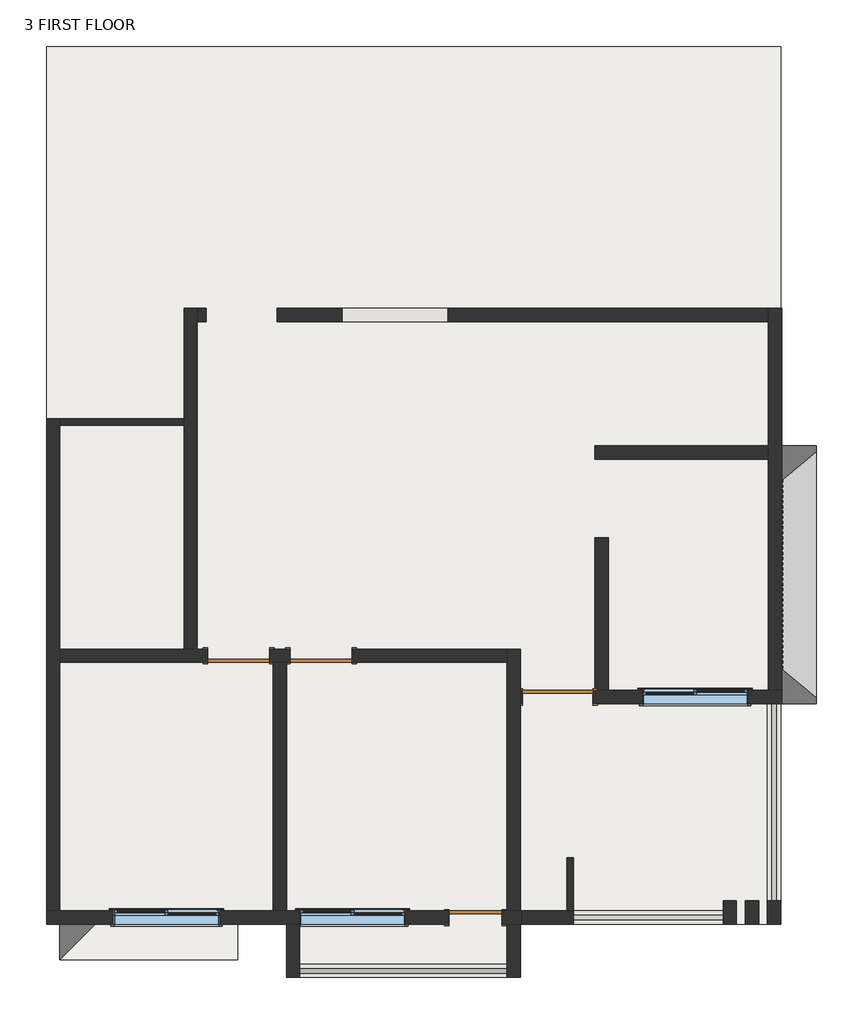
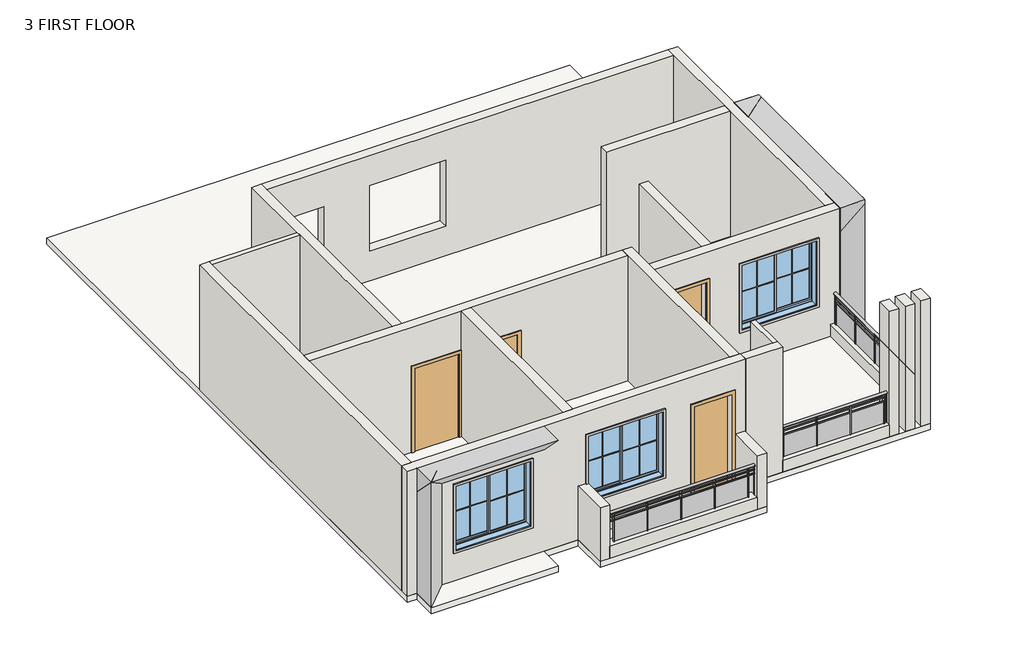
# One storey: 22 walls, 14 proxies, 4 doors, 3 railings, 3 windows, 1 slab.
"""IFC4 building model written with IfcOpenShell, lengths in millimetres."""

from ifc_helpers import new_model, si_unit, point, frame, origin, place, context, project, spatial, polyline, ellipse_curve, trimmed, outline, extrude, faceted_brep, transform, mapped, element, save
from ifc_brep_helpers import plane_surface, extruded_surface, advanced_brep
from components import generic_models_2_generic_models_2_bb9d770e, generic_models_4_generic_models_4_3dac0b09, muntin_pattern_2x2_muntin_pattern_2x2_52b72501, muntin_pattern_2x2_muntin_pattern_2x2_a6e57790, trim_window_exterior_flat_with_sill_c98b2dec, trim_window_exterior_flat_with_sill_2360300c, trim_window_interior_flat_picture_frame_b05ee221, trim_window_interior_flat_picture_frame_67c405d8, single_flush_9d399b00, single_flush_0848dd25, single_flush_md_e3fbe821, single_flush_md_2_408f135a, window_sliding_double_89c6b595, window_sliding_double_c634d93e

model = new_model("IFC4")

# Units and contexts
model_context = context("Model", 3, world=origin())
ifc_project = project(units=[si_unit("LENGTHUNIT", "METRE", prefix="MILLI")], contexts=[model_context])

# Site, building, storey
site = spatial("IfcSite", under=ifc_project)
building = spatial("IfcBuilding", under=site)
storey = spatial("IfcBuildingStorey", under=building, Name="3 FIRST FLOOR", Elevation=3505.2)

# Proxies
placement = place(None, origin())
generic_models_2_generic_models_2_shape = generic_models_2_generic_models_2_bb9d770e(model_context)
element("IfcBuildingElementProxy", 1, Name="Generic Models 2 : Generic Models 2", ObjectType="Generic Models 2 : Generic Models 2", at=placement, inside=storey, context=model_context, shape_type="MappedRepresentation", body=[
    mapped(generic_models_2_generic_models_2_shape, transform((0.0, 0.0, 0.0), x_axis=(1.0, 0.0, 0.0), y_axis=(0.0, 1.0, 0.0), z_axis=(0.0, 0.0, 1.0))),
])
generic_models_4_generic_models_4_shape = generic_models_4_generic_models_4_3dac0b09(model_context)
element("IfcBuildingElementProxy", 2, Name="Generic Models 4 : Generic Models 4", ObjectType="Generic Models 4 : Generic Models 4", at=placement, inside=storey, context=model_context, shape_type="MappedRepresentation", body=[
    mapped(generic_models_4_generic_models_4_shape, transform((0.0, 0.0, 0.0), x_axis=(1.0, 0.0, 0.0), y_axis=(0.0, 1.0, 0.0), z_axis=(0.0, 0.0, 1.0))),
])
muntin_pattern_2x2_muntin_pattern_2x2_shape = muntin_pattern_2x2_muntin_pattern_2x2_52b72501(model_context)
element("IfcBuildingElementProxy", 3, Name="Muntin Pattern_2x2 : Muntin Pattern_2x2", ObjectType="Muntin Pattern_2x2 : Muntin Pattern_2x2", at=placement, inside=storey, context=model_context, shape_type="MappedRepresentation", body=[
    mapped(muntin_pattern_2x2_muntin_pattern_2x2_shape, transform((-2582.8521564, -7786.433484, 4349.75), x_axis=(1.0, 0.0, 0.0), y_axis=(0.0, 1.0, 0.0), z_axis=(0.0, 0.0, 1.0))),
])
element("IfcBuildingElementProxy", 4, Name="Muntin Pattern_2x2 : Muntin Pattern_2x2", ObjectType="Muntin Pattern_2x2 : Muntin Pattern_2x2", at=placement, inside=storey, context=model_context, shape_type="MappedRepresentation", body=[
    mapped(muntin_pattern_2x2_muntin_pattern_2x2_shape, transform((-3455.9771564, -7741.983484, 4349.75), x_axis=(1.0, 0.0, 0.0), y_axis=(0.0, 1.0, 0.0), z_axis=(0.0, 0.0, 1.0))),
])
element("IfcBuildingElementProxy", 5, Name="Muntin Pattern_2x2 : Muntin Pattern_2x2", ObjectType="Muntin Pattern_2x2 : Muntin Pattern_2x2", at=placement, inside=storey, context=model_context, shape_type="MappedRepresentation", body=[
    mapped(muntin_pattern_2x2_muntin_pattern_2x2_shape, transform((618.6182451, -7786.433484, 4502.15), x_axis=(1.0, 0.0, 0.0), y_axis=(0.0, 1.0, 0.0), z_axis=(0.0, 0.0, 1.0))),
])
element("IfcBuildingElementProxy", 6, Name="Muntin Pattern_2x2 : Muntin Pattern_2x2", ObjectType="Muntin Pattern_2x2 : Muntin Pattern_2x2", at=placement, inside=storey, context=model_context, shape_type="MappedRepresentation", body=[
    mapped(muntin_pattern_2x2_muntin_pattern_2x2_shape, transform((-254.5067549, -7741.983484, 4502.15), x_axis=(1.0, 0.0, 0.0), y_axis=(0.0, 1.0, 0.0), z_axis=(0.0, 0.0, 1.0))),
])
muntin_pattern_2x2_muntin_pattern_2x2_2_shape = muntin_pattern_2x2_muntin_pattern_2x2_a6e57790(model_context)
element("IfcBuildingElementProxy", 7, Name="Muntin Pattern_2x2 : Muntin Pattern_2x2", ObjectType="Muntin Pattern_2x2 : Muntin Pattern_2x2", at=placement, inside=storey, context=model_context, shape_type="MappedRepresentation", body=[
    mapped(muntin_pattern_2x2_muntin_pattern_2x2_2_shape, transform((5644.6432451, -3992.2046941, 4502.15), x_axis=(-1.0, 0.0, 0.0), y_axis=(0.0, -1.0, 0.0), z_axis=(0.0, 0.0, 1.0))),
])
element("IfcBuildingElementProxy", 8, Name="Muntin Pattern_2x2 : Muntin Pattern_2x2", ObjectType="Muntin Pattern_2x2 : Muntin Pattern_2x2", at=placement, inside=storey, context=model_context, shape_type="MappedRepresentation", body=[
    mapped(muntin_pattern_2x2_muntin_pattern_2x2_2_shape, transform((6517.7682451, -3947.7546941, 4502.15), x_axis=(-1.0, 0.0, 0.0), y_axis=(0.0, -1.0, 0.0), z_axis=(0.0, 0.0, 1.0))),
])
trim_window_exterior_flat_with_sill_shape = trim_window_exterior_flat_with_sill_c98b2dec(model_context)
element("IfcBuildingElementProxy", 9, Name="Trim-Window-Exterior-Flat : with Sill", ObjectType="Trim-Window-Exterior-Flat : with Sill", at=placement, inside=storey, context=model_context, shape_type="MappedRepresentation", body=[
    mapped(trim_window_exterior_flat_with_sill_shape, transform((-3019.4146564, -7732.458484, 5943.6), x_axis=(-1.0, 0.0, 0.0), y_axis=(0.0, 0.0, 1.0), z_axis=(0.0, 1.0, 0.0))),
])
element("IfcBuildingElementProxy", 10, Name="Trim-Window-Exterior-Flat : with Sill", ObjectType="Trim-Window-Exterior-Flat : with Sill", at=placement, inside=storey, context=model_context, shape_type="MappedRepresentation", body=[
    mapped(trim_window_exterior_flat_with_sill_shape, transform((182.0557451, -7732.458484, 6096.0), x_axis=(-1.0, 0.0, 0.0), y_axis=(0.0, 0.0, 1.0), z_axis=(0.0, 1.0, 0.0))),
])
trim_window_exterior_flat_with_sill_2_shape = trim_window_exterior_flat_with_sill_2360300c(model_context)
element("IfcBuildingElementProxy", 11, Name="Trim-Window-Exterior-Flat : with Sill", ObjectType="Trim-Window-Exterior-Flat : with Sill", at=placement, inside=storey, context=model_context, shape_type="MappedRepresentation", body=[
    mapped(trim_window_exterior_flat_with_sill_2_shape, transform((6081.2057451, -3938.2296941, 6096.0), x_axis=(1.0, 0.0, 0.0), y_axis=(0.0, 0.0, -1.0), z_axis=(0.0, 1.0, 0.0))),
])
trim_window_interior_flat_picture_frame_shape = trim_window_interior_flat_picture_frame_b05ee221(model_context)
element("IfcBuildingElementProxy", 12, Name="Trim-Window-Interior-Flat : Picture Frame", ObjectType="Trim-Window-Interior-Flat : Picture Frame", at=placement, inside=storey, context=model_context, shape_type="MappedRepresentation", body=[
    mapped(trim_window_interior_flat_picture_frame_shape, transform((-3019.4146564, -7961.058484, 5943.6), x_axis=(1.0, 0.0, 0.0), y_axis=(0.0, 0.0, 1.0), z_axis=(0.0, -1.0, 0.0))),
])
element("IfcBuildingElementProxy", 13, Name="Trim-Window-Interior-Flat : Picture Frame", ObjectType="Trim-Window-Interior-Flat : Picture Frame", at=placement, inside=storey, context=model_context, shape_type="MappedRepresentation", body=[
    mapped(trim_window_interior_flat_picture_frame_shape, transform((182.0557451, -7961.058484, 6096.0), x_axis=(1.0, 0.0, 0.0), y_axis=(0.0, 0.0, 1.0), z_axis=(0.0, -1.0, 0.0))),
])
trim_window_interior_flat_picture_frame_2_shape = trim_window_interior_flat_picture_frame_67c405d8(model_context)
element("IfcBuildingElementProxy", 14, Name="Trim-Window-Interior-Flat : Picture Frame", ObjectType="Trim-Window-Interior-Flat : Picture Frame", at=placement, inside=storey, context=model_context, shape_type="MappedRepresentation", body=[
    mapped(trim_window_interior_flat_picture_frame_2_shape, transform((6081.2057451, -4166.8296941, 6096.0), x_axis=(-1.0, 0.0, 0.0), y_axis=(0.0, 0.0, -1.0), z_axis=(0.0, -1.0, 0.0))),
])

# Doors
single_flush_shape = single_flush_9d399b00(model_context)
element("IfcDoor", 15, ObjectType="Single-Flush", at=placement, inside=storey, context=model_context, shape_type="MappedRepresentation", body=[
    mapped(single_flush_shape, transform((-357.6942549, -3341.3296941, 3505.2), x_axis=(-1.0, 0.0, 0.0), y_axis=(0.0, -1.0, 0.0), z_axis=(0.0, 0.0, 1.0))),
])
single_flush_2_shape = single_flush_0848dd25(model_context)
element("IfcDoor", 16, ObjectType="Single-Flush", at=placement, inside=storey, context=model_context, shape_type="MappedRepresentation", body=[
    mapped(single_flush_2_shape, transform((-1780.0942549, -3341.3296941, 3505.2), x_axis=(1.0, 0.0, 0.0), y_axis=(0.0, 1.0, 0.0), z_axis=(0.0, 0.0, 1.0))),
])
single_flush_md_shape = single_flush_md_e3fbe821(model_context)
element("IfcDoor", 17, ObjectType="Single-Flush : MD", at=placement, inside=storey, context=model_context, shape_type="MappedRepresentation", body=[
    mapped(single_flush_md_shape, transform((3712.6557451, -4052.5296941, 3505.2), x_axis=(1.0, 0.0, 0.0), y_axis=(0.0, 1.0, 0.0), z_axis=(0.0, 0.0, 1.0))),
])
single_flush_md_2_shape = single_flush_md_2_408f135a(model_context)
element("IfcDoor", 18, ObjectType="Single-Flush : MD 2", at=placement, inside=storey, context=model_context, shape_type="MappedRepresentation", body=[
    mapped(single_flush_md_2_shape, transform((2296.6057451, -7846.758484, 3505.2), x_axis=(1.0, 0.0, 0.0), y_axis=(0.0, 1.0, 0.0), z_axis=(0.0, 0.0, 1.0))),
])

# Railings
element("IfcRailing", 19, ObjectType="Glass Panel - Bottom Fill", at=placement, inside=storey, context=model_context, shape_type="SolidModel", body=[
    advanced_brep(
    [(-725.9942549, -8723.058484, 4572.0), (-725.9942549, -8799.258484, 4572.0), (2842.7057451, -8723.058484, 4572.0), (2842.7057451, -8799.258484, 4572.0)],
    [
        (0, 1, ellipse_curve(frame((-725.9942549, -8761.158484, 4572.0), z_axis=(-1.0, 0.0, 0.0), x_axis=(0.0, -1.0, 0.0)), 38.1, 28.575)),
        (1, 0, ellipse_curve(frame((-725.9942549, -8761.158484, 4572.0), z_axis=(-1.0, 0.0, 0.0), x_axis=(0.0, -1.0, 0.0)), 38.1, 28.575)),
        (2, 3, ellipse_curve(frame((2842.7057451, -8761.158484, 4572.0), z_axis=(1.0, 0.0, 0.0), x_axis=(0.0, -1.0, 0.0)), 38.1, 28.575)),
        (3, 2, ellipse_curve(frame((2842.7057451, -8761.158484, 4572.0), z_axis=(1.0, 0.0, 0.0), x_axis=(0.0, -1.0, 0.0)), 38.1, 28.575)),
        (0, 2),
        (3, 1),
    ],
    [
        plane_surface(frame((-725.9942549, -8761.158484, 4572.0), z_axis=(-1.0, 0.0, 0.0), x_axis=(0.0, 1.0, 0.0))),
        plane_surface(frame((2842.7057451, -8761.158484, 4572.0), z_axis=(1.0, 0.0, 0.0), x_axis=(0.0, 1.0, 0.0))),
        extruded_surface(trimmed(ellipse_curve(frame((2842.7057451, -8761.158484, 4572.0), z_axis=(-1.0, 0.0, 0.0), x_axis=(0.0, -1.0, 0.0)), 38.1, 28.575), [point((2842.7057451, -8723.058484, 4572.0))], [point((2842.7057451, -8799.258484, 4572.0))], True, "CARTESIAN"), (-3568.7, 0.0, 0.0), 3568.7),
        extruded_surface(trimmed(ellipse_curve(frame((2842.7057451, -8761.158484, 4572.0), z_axis=(-1.0, 0.0, 0.0), x_axis=(0.0, -1.0, 0.0)), 38.1, 28.575), [point((2842.7057451, -8799.258484, 4572.0))], [point((2842.7057451, -8723.058484, 4572.0))], True, "CARTESIAN"), (-3568.7, 0.0, 0.0), 3568.7),
    ],
    [
        (0, [[1, 2]]),
        (1, [[3, 4]]),
        (2, [[-1, 5, -4, 6]]),
        (3, [[-2, -6, -3, -5]]),
    ],
),
    extrude(outline(polyline([(-725.9942549, -8773.858484), (-725.9942549, -8748.458484), (2842.7057451, -8748.458484), (2842.7057451, -8773.858484), (-725.9942549, -8773.858484)])), frame((0.0, 0.0, 4457.7), z_axis=(0.0, 0.0, 1.0), x_axis=(1.0, 0.0, 0.0)), (0.0, 0.0, 1.0), 25.4),
    extrude(outline(polyline([(-725.9942549, -8773.858484), (-725.9942549, -8748.458484), (2842.7057451, -8748.458484), (2842.7057451, -8773.858484), (-725.9942549, -8773.858484)])), frame((0.0, 0.0, 4356.1), z_axis=(0.0, 0.0, 1.0), x_axis=(1.0, 0.0, 0.0)), (0.0, 0.0, 1.0), 25.4),
    extrude(outline(polyline([(2677.6057451, -8786.558484), (2677.6057451, -8735.758484), (2690.3057451, -8735.758484), (2690.3057451, -8786.558484), (2677.6057451, -8786.558484)])), frame((0.0, 0.0, 3657.6), z_axis=(0.0, 0.0, 1.0), x_axis=(1.0, 0.0, 0.0)), (0.0, 0.0, 1.0), 885.825),
    extrude(outline(polyline([(1871.1557451, -8754.623327), (2683.9557451, -8754.623327), (2683.9557451, -8760.973327), (1871.1557451, -8760.973327), (1871.1557451, -8754.623327)])), frame((0.0, 0.0, 3759.2), z_axis=(0.0, 0.0, 1.0), x_axis=(1.0, 0.0, 0.0)), (0.0, 0.0, 1.0), 596.9),
    extrude(outline(polyline([(1864.8057451, -8786.558484), (1864.8057451, -8735.758484), (1877.5057451, -8735.758484), (1877.5057451, -8786.558484), (1864.8057451, -8786.558484)])), frame((0.0, 0.0, 3657.6), z_axis=(0.0, 0.0, 1.0), x_axis=(1.0, 0.0, 0.0)), (0.0, 0.0, 1.0), 885.825),
    extrude(outline(polyline([(1058.3557451, -8754.623327), (1871.1557451, -8754.623327), (1871.1557451, -8760.973327), (1058.3557451, -8760.973327), (1058.3557451, -8754.623327)])), frame((0.0, 0.0, 3759.2), z_axis=(0.0, 0.0, 1.0), x_axis=(1.0, 0.0, 0.0)), (0.0, 0.0, 1.0), 596.9),
    extrude(outline(polyline([(1052.0057451, -8786.558484), (1052.0057451, -8735.758484), (1064.7057451, -8735.758484), (1064.7057451, -8786.558484), (1052.0057451, -8786.558484)])), frame((0.0, 0.0, 3657.6), z_axis=(0.0, 0.0, 1.0), x_axis=(1.0, 0.0, 0.0)), (0.0, 0.0, 1.0), 885.825),
    extrude(outline(polyline([(245.5557451, -8754.623327), (1058.3557451, -8754.623327), (1058.3557451, -8760.973327), (245.5557451, -8760.973327), (245.5557451, -8754.623327)])), frame((0.0, 0.0, 3759.2), z_axis=(0.0, 0.0, 1.0), x_axis=(1.0, 0.0, 0.0)), (0.0, 0.0, 1.0), 596.9),
    extrude(outline(polyline([(239.2057451, -8786.558484), (239.2057451, -8735.758484), (251.9057451, -8735.758484), (251.9057451, -8786.558484), (239.2057451, -8786.558484)])), frame((0.0, 0.0, 3657.6), z_axis=(0.0, 0.0, 1.0), x_axis=(1.0, 0.0, 0.0)), (0.0, 0.0, 1.0), 885.825),
    extrude(outline(polyline([(-567.2442549, -8754.623327), (245.5557451, -8754.623327), (245.5557451, -8760.973327), (-567.2442549, -8760.973327), (-567.2442549, -8754.623327)])), frame((0.0, 0.0, 3759.2), z_axis=(0.0, 0.0, 1.0), x_axis=(1.0, 0.0, 0.0)), (0.0, 0.0, 1.0), 596.9),
    extrude(outline(polyline([(-573.5942549, -8786.558484), (-573.5942549, -8735.758484), (-560.8942549, -8735.758484), (-560.8942549, -8786.558484), (-573.5942549, -8786.558484)])), frame((0.0, 0.0, 3657.6), z_axis=(0.0, 0.0, 1.0), x_axis=(1.0, 0.0, 0.0)), (0.0, 0.0, 1.0), 885.825),
    extrude(outline(polyline([(2830.0057451, -8770.683484), (2830.0057451, -8751.633484), (2849.0557451, -8751.633484), (2849.0557451, -8770.683484), (2830.0057451, -8770.683484)])), frame((0.0, 0.0, 3657.6), z_axis=(0.0, 0.0, 1.0), x_axis=(1.0, 0.0, 0.0)), (0.0, 0.0, 1.0), 885.825),
    extrude(outline(polyline([(-732.3442549, -8770.683484), (-732.3442549, -8751.633484), (-713.2942549, -8751.633484), (-713.2942549, -8770.683484), (-732.3442549, -8770.683484)])), frame((0.0, 0.0, 3657.6), z_axis=(0.0, 0.0, 1.0), x_axis=(1.0, 0.0, 0.0)), (0.0, 0.0, 1.0), 885.825),
])
element("IfcRailing", 20, ObjectType="Glass Panel - Bottom Fill", at=placement, inside=storey, context=model_context, shape_type="SolidModel", body=[
    advanced_brep(
    [(7400.6590234, -7554.658484, 4572.0), (7476.8590234, -7554.658484, 4572.0), (7400.6590234, -4166.8296941, 4572.0), (7476.8590234, -4166.8296941, 4572.0)],
    [
        (0, 1, ellipse_curve(frame((7438.7590234, -7554.658484, 4572.0), z_axis=(0.0, -1.0, 0.0), x_axis=(1.0, 0.0, 0.0)), 38.1, 28.575)),
        (1, 0, ellipse_curve(frame((7438.7590234, -7554.658484, 4572.0), z_axis=(0.0, -1.0, 0.0), x_axis=(1.0, 0.0, 0.0)), 38.1, 28.575)),
        (2, 3, ellipse_curve(frame((7438.7590234, -4166.8296941, 4572.0), z_axis=(0.0, 1.0, 0.0), x_axis=(1.0, 0.0, 0.0)), 38.1, 28.575)),
        (3, 2, ellipse_curve(frame((7438.7590234, -4166.8296941, 4572.0), z_axis=(0.0, 1.0, 0.0), x_axis=(1.0, 0.0, 0.0)), 38.1, 28.575)),
        (0, 2),
        (3, 1),
    ],
    [
        plane_surface(frame((7438.7590234, -7554.658484, 4572.0), z_axis=(0.0, -1.0, 0.0), x_axis=(0.0, 0.0, 1.0))),
        plane_surface(frame((7438.7590234, -4166.8296941, 4572.0), z_axis=(0.0, 1.0, 0.0), x_axis=(0.0, 0.0, 1.0))),
        extruded_surface(trimmed(ellipse_curve(frame((7438.7590234, -4166.8296941, 4572.0), z_axis=(0.0, -1.0, 0.0), x_axis=(1.0, 0.0, 0.0)), 38.1, 28.575), [point((7400.6590234, -4166.8296941, 4572.0))], [point((7476.8590234, -4166.8296941, 4572.0))], True, "CARTESIAN"), (0.0, -3387.8287898999997, 0.0), 3387.8287898999997),
        extruded_surface(trimmed(ellipse_curve(frame((7438.7590234, -4166.8296941, 4572.0), z_axis=(0.0, -1.0, 0.0), x_axis=(1.0, 0.0, 0.0)), 38.1, 28.575), [point((7476.8590234, -4166.8296941, 4572.0))], [point((7400.6590234, -4166.8296941, 4572.0))], True, "CARTESIAN"), (0.0, -3387.8287898999997, 0.0), 3387.8287898999997),
    ],
    [
        (0, [[1, 2]]),
        (1, [[3, 4]]),
        (2, [[-1, 5, -4, 6]]),
        (3, [[-2, -6, -3, -5]]),
    ],
),
    extrude(outline(polyline([(7451.4590234, -7554.658484), (7426.0590234, -7554.658484), (7426.0590234, -4166.8296941), (7451.4590234, -4166.8296941), (7451.4590234, -7554.658484)])), frame((0.0, 0.0, 4457.7), z_axis=(0.0, 0.0, 1.0), x_axis=(1.0, 0.0, 0.0)), (0.0, 0.0, 1.0), 25.4),
    extrude(outline(polyline([(7451.4590234, -7554.658484), (7426.0590234, -7554.658484), (7426.0590234, -4166.8296941), (7451.4590234, -4166.8296941), (7451.4590234, -7554.658484)])), frame((0.0, 0.0, 4356.1), z_axis=(0.0, 0.0, 1.0), x_axis=(1.0, 0.0, 0.0)), (0.0, 0.0, 1.0), 25.4),
    extrude(outline(polyline([(7464.1590234, -4241.4940891), (7413.3590234, -4241.4940891), (7413.3590234, -4228.7940891), (7464.1590234, -4228.7940891), (7464.1590234, -4241.4940891)])), frame((0.0, 0.0, 3657.6), z_axis=(0.0, 0.0, 1.0), x_axis=(1.0, 0.0, 0.0)), (0.0, 0.0, 1.0), 885.825),
    extrude(outline(polyline([(7432.2238664, -5047.9440891), (7432.2238664, -4235.1440891), (7438.5738664, -4235.1440891), (7438.5738664, -5047.9440891), (7432.2238664, -5047.9440891)])), frame((0.0, 0.0, 3759.2), z_axis=(0.0, 0.0, 1.0), x_axis=(1.0, 0.0, 0.0)), (0.0, 0.0, 1.0), 596.9),
    extrude(outline(polyline([(7464.1590234, -5054.2940891), (7413.3590234, -5054.2940891), (7413.3590234, -5041.5940891), (7464.1590234, -5041.5940891), (7464.1590234, -5054.2940891)])), frame((0.0, 0.0, 3657.6), z_axis=(0.0, 0.0, 1.0), x_axis=(1.0, 0.0, 0.0)), (0.0, 0.0, 1.0), 885.825),
    extrude(outline(polyline([(7432.2238664, -5860.7440891), (7432.2238664, -5047.9440891), (7438.5738664, -5047.9440891), (7438.5738664, -5860.7440891), (7432.2238664, -5860.7440891)])), frame((0.0, 0.0, 3759.2), z_axis=(0.0, 0.0, 1.0), x_axis=(1.0, 0.0, 0.0)), (0.0, 0.0, 1.0), 596.9),
    extrude(outline(polyline([(7464.1590234, -5867.0940891), (7413.3590234, -5867.0940891), (7413.3590234, -5854.3940891), (7464.1590234, -5854.3940891), (7464.1590234, -5867.0940891)])), frame((0.0, 0.0, 3657.6), z_axis=(0.0, 0.0, 1.0), x_axis=(1.0, 0.0, 0.0)), (0.0, 0.0, 1.0), 885.825),
    extrude(outline(polyline([(7432.2238664, -6673.5440891), (7432.2238664, -5860.7440891), (7438.5738664, -5860.7440891), (7438.5738664, -6673.5440891), (7432.2238664, -6673.5440891)])), frame((0.0, 0.0, 3759.2), z_axis=(0.0, 0.0, 1.0), x_axis=(1.0, 0.0, 0.0)), (0.0, 0.0, 1.0), 596.9),
    extrude(outline(polyline([(7464.1590234, -6679.8940891), (7413.3590234, -6679.8940891), (7413.3590234, -6667.1940891), (7464.1590234, -6667.1940891), (7464.1590234, -6679.8940891)])), frame((0.0, 0.0, 3657.6), z_axis=(0.0, 0.0, 1.0), x_axis=(1.0, 0.0, 0.0)), (0.0, 0.0, 1.0), 885.825),
    extrude(outline(polyline([(7432.2238664, -7486.3440891), (7432.2238664, -6673.5440891), (7438.5738664, -6673.5440891), (7438.5738664, -7486.3440891), (7432.2238664, -7486.3440891)])), frame((0.0, 0.0, 3759.2), z_axis=(0.0, 0.0, 1.0), x_axis=(1.0, 0.0, 0.0)), (0.0, 0.0, 1.0), 596.9),
    extrude(outline(polyline([(7464.1590234, -7492.6940891), (7413.3590234, -7492.6940891), (7413.3590234, -7479.9940891), (7464.1590234, -7479.9940891), (7464.1590234, -7492.6940891)])), frame((0.0, 0.0, 3657.6), z_axis=(0.0, 0.0, 1.0), x_axis=(1.0, 0.0, 0.0)), (0.0, 0.0, 1.0), 885.825),
    extrude(outline(polyline([(7448.2840234, -4179.5296941), (7429.2340234, -4179.5296941), (7429.2340234, -4160.4796941), (7448.2840234, -4160.4796941), (7448.2840234, -4179.5296941)])), frame((0.0, 0.0, 3657.6), z_axis=(0.0, 0.0, 1.0), x_axis=(1.0, 0.0, 0.0)), (0.0, 0.0, 1.0), 885.825),
    extrude(outline(polyline([(7448.2840234, -7561.008484), (7429.2340234, -7561.008484), (7429.2340234, -7541.958484), (7448.2840234, -7541.958484), (7448.2840234, -7561.008484)])), frame((0.0, 0.0, 3657.6), z_axis=(0.0, 0.0, 1.0), x_axis=(1.0, 0.0, 0.0)), (0.0, 0.0, 1.0), 885.825),
])
element("IfcRailing", 21, ObjectType="Glass Panel - Bottom Fill", at=placement, inside=storey, context=model_context, shape_type="SolidModel", body=[
    advanced_brep(
    [(6562.4590234, -7884.858484, 4572.0), (6562.4590234, -7808.658484, 4572.0), (3985.7057451, -7884.858484, 4572.0), (3985.7057451, -7808.658484, 4572.0)],
    [
        (0, 1, ellipse_curve(frame((6562.4590234, -7846.758484, 4572.0), z_axis=(1.0, 0.0, 0.0), x_axis=(0.0, 1.0, 0.0)), 38.1, 28.575)),
        (1, 0, ellipse_curve(frame((6562.4590234, -7846.758484, 4572.0), z_axis=(1.0, 0.0, 0.0), x_axis=(0.0, 1.0, 0.0)), 38.1, 28.575)),
        (2, 3, ellipse_curve(frame((3985.7057451, -7846.758484, 4572.0), z_axis=(-1.0, 0.0, 0.0), x_axis=(0.0, 1.0, 0.0)), 38.1, 28.575)),
        (3, 2, ellipse_curve(frame((3985.7057451, -7846.758484, 4572.0), z_axis=(-1.0, 0.0, 0.0), x_axis=(0.0, 1.0, 0.0)), 38.1, 28.575)),
        (0, 2),
        (3, 1),
    ],
    [
        plane_surface(frame((6562.4590234, -7846.758484, 4572.0), z_axis=(1.0, 0.0, 0.0), x_axis=(0.0, -1.0, 0.0))),
        plane_surface(frame((3985.7057451, -7846.758484, 4572.0), z_axis=(-1.0, 0.0, 0.0), x_axis=(0.0, -1.0, 0.0))),
        extruded_surface(trimmed(ellipse_curve(frame((3985.7057451, -7846.758484, 4572.0), z_axis=(1.0, 0.0, 0.0), x_axis=(0.0, 1.0, 0.0)), 38.1, 28.575), [point((3985.7057451, -7884.858484, 4572.0))], [point((3985.7057451, -7808.658484, 4572.0))], True, "CARTESIAN"), (2576.7532782999997, 0.0, 0.0), 2576.7532782999997),
        extruded_surface(trimmed(ellipse_curve(frame((3985.7057451, -7846.758484, 4572.0), z_axis=(1.0, 0.0, 0.0), x_axis=(0.0, 1.0, 0.0)), 38.1, 28.575), [point((3985.7057451, -7808.658484, 4572.0))], [point((3985.7057451, -7884.858484, 4572.0))], True, "CARTESIAN"), (2576.7532782999997, 0.0, 0.0), 2576.7532782999997),
    ],
    [
        (0, [[1, 2]]),
        (1, [[3, 4]]),
        (2, [[-1, 5, -4, 6]]),
        (3, [[-2, -6, -3, -5]]),
    ],
),
    extrude(outline(polyline([(6562.4590234, -7834.058484), (6562.4590234, -7859.458484), (3985.7057451, -7859.458484), (3985.7057451, -7834.058484), (6562.4590234, -7834.058484)])), frame((0.0, 0.0, 4457.7), z_axis=(0.0, 0.0, 1.0), x_axis=(1.0, 0.0, 0.0)), (0.0, 0.0, 1.0), 25.4),
    extrude(outline(polyline([(6562.4590234, -7834.058484), (6562.4590234, -7859.458484), (3985.7057451, -7859.458484), (3985.7057451, -7834.058484), (6562.4590234, -7834.058484)])), frame((0.0, 0.0, 4356.1), z_axis=(0.0, 0.0, 1.0), x_axis=(1.0, 0.0, 0.0)), (0.0, 0.0, 1.0), 25.4),
    extrude(outline(polyline([(4061.2323842, -7821.358484), (4061.2323842, -7872.158484), (4048.5323842, -7872.158484), (4048.5323842, -7821.358484), (4061.2323842, -7821.358484)])), frame((0.0, 0.0, 3657.6), z_axis=(0.0, 0.0, 1.0), x_axis=(1.0, 0.0, 0.0)), (0.0, 0.0, 1.0), 885.825),
    extrude(outline(polyline([(4867.6823842, -7853.293641), (4054.8823842, -7853.293641), (4054.8823842, -7846.943641), (4867.6823842, -7846.943641), (4867.6823842, -7853.293641)])), frame((0.0, 0.0, 3759.2), z_axis=(0.0, 0.0, 1.0), x_axis=(1.0, 0.0, 0.0)), (0.0, 0.0, 1.0), 596.9),
    extrude(outline(polyline([(4874.0323842, -7821.358484), (4874.0323842, -7872.158484), (4861.3323842, -7872.158484), (4861.3323842, -7821.358484), (4874.0323842, -7821.358484)])), frame((0.0, 0.0, 3657.6), z_axis=(0.0, 0.0, 1.0), x_axis=(1.0, 0.0, 0.0)), (0.0, 0.0, 1.0), 885.825),
    extrude(outline(polyline([(5680.4823842, -7853.293641), (4867.6823842, -7853.293641), (4867.6823842, -7846.943641), (5680.4823842, -7846.943641), (5680.4823842, -7853.293641)])), frame((0.0, 0.0, 3759.2), z_axis=(0.0, 0.0, 1.0), x_axis=(1.0, 0.0, 0.0)), (0.0, 0.0, 1.0), 596.9),
    extrude(outline(polyline([(5686.8323842, -7821.358484), (5686.8323842, -7872.158484), (5674.1323842, -7872.158484), (5674.1323842, -7821.358484), (5686.8323842, -7821.358484)])), frame((0.0, 0.0, 3657.6), z_axis=(0.0, 0.0, 1.0), x_axis=(1.0, 0.0, 0.0)), (0.0, 0.0, 1.0), 885.825),
    extrude(outline(polyline([(6493.2823842, -7853.293641), (5680.4823842, -7853.293641), (5680.4823842, -7846.943641), (6493.2823842, -7846.943641), (6493.2823842, -7853.293641)])), frame((0.0, 0.0, 3759.2), z_axis=(0.0, 0.0, 1.0), x_axis=(1.0, 0.0, 0.0)), (0.0, 0.0, 1.0), 596.9),
    extrude(outline(polyline([(6499.6323842, -7821.358484), (6499.6323842, -7872.158484), (6486.9323842, -7872.158484), (6486.9323842, -7821.358484), (6499.6323842, -7821.358484)])), frame((0.0, 0.0, 3657.6), z_axis=(0.0, 0.0, 1.0), x_axis=(1.0, 0.0, 0.0)), (0.0, 0.0, 1.0), 885.825),
    extrude(outline(polyline([(3998.4057451, -7837.233484), (3998.4057451, -7856.283484), (3979.3557451, -7856.283484), (3979.3557451, -7837.233484), (3998.4057451, -7837.233484)])), frame((0.0, 0.0, 3657.6), z_axis=(0.0, 0.0, 1.0), x_axis=(1.0, 0.0, 0.0)), (0.0, 0.0, 1.0), 885.825),
    extrude(outline(polyline([(6568.8090234, -7837.233484), (6568.8090234, -7856.283484), (6549.7590234, -7856.283484), (6549.7590234, -7837.233484), (6568.8090234, -7837.233484)])), frame((0.0, 0.0, 3657.6), z_axis=(0.0, 0.0, 1.0), x_axis=(1.0, 0.0, 0.0)), (0.0, 0.0, 1.0), 885.825),
])

# Slab
element("IfcSlab", 22, ObjectType="ROOF", at=placement, inside=storey, context=model_context, shape_type="SweptSolid", body=[
    extrude(outline(polyline([(7553.0590234, 7136.1703059), (7553.0590234, 267.4142537), (8162.6590234, 267.4142537), (8162.6590234, -4166.8296941), (7553.0590234, -4166.8296941), (7553.0590234, -7961.058484), (3071.3057451, -7961.058484), (3071.3057451, -8875.458484), (-954.5942549, -8875.458484), (-954.5942549, -7961.058484), (-1792.7942549, -7961.058484), (-1792.7942549, -8570.658484), (-4855.6350579, -8570.658484), (-4855.6350579, -7961.058484), (-5084.2350579, -7961.058484), (-5084.2350579, 7136.1703059), (7553.0590234, 7136.1703059)])), frame((0.0, 0.0, 3352.8), z_axis=(0.0, 0.0, 1.0), x_axis=(1.0, 0.0, 0.0)), (0.0, 0.0, 1.0), 152.4),
])

# Walls
element("IfcWall", 23, ObjectType="4.5\"", at=placement, inside=storey, context=model_context, shape_type="SweptSolid", body=[
    extrude(outline(polyline([(-2719.8942549, 618.9452215), (-4855.6350579, 618.9452215), (-4855.6350579, 733.2452215), (-2719.8942549, 733.2452215), (-2719.8942549, 618.9452215)])), frame((0.0, 0.0, 3505.2), z_axis=(0.0, 0.0, 1.0), x_axis=(1.0, 0.0, 0.0)), (0.0, 0.0, 1.0), 3200.4),
])
element("IfcWall", 24, ObjectType="4.5\"", at=placement, inside=storey, context=model_context, shape_type="SweptSolid", body=[
    extrude(outline(polyline([(3985.7057451, -6818.058484), (3985.7057451, -7732.458484), (3871.4057451, -7732.458484), (3871.4057451, -6818.058484), (3985.7057451, -6818.058484)])), frame((0.0, 0.0, 3505.2), z_axis=(0.0, 0.0, 1.0), x_axis=(1.0, 0.0, 0.0)), (0.0, 0.0, 1.0), 3200.4),
])
element("IfcWall", 25, ObjectType="9\"", at=placement, inside=storey, context=model_context, shape_type="Brep", body=[
    faceted_brep([(2753.8057451, -7961.058484, 5943.6), (2753.8057451, -7961.058484, 3505.2), (2842.7057451, -7961.058484, 3505.2), (3071.3057451, -7961.058484, 3505.2), (3090.3557451, -7961.058484, 3505.2), (3090.3557451, -7961.058484, 6705.6), (-5084.2350579, -7961.058484, 6705.6), (-5084.2350579, -7961.058484, 3505.2), (-954.5942549, -7961.058484, 3505.2), (-725.9942549, -7961.058484, 3505.2), (1839.4057451, -7961.058484, 3505.2), (1839.4057451, -7961.058484, 5943.6), (-2105.0146564, -7961.058484, 5943.6), (-2105.0146564, -7961.058484, 4267.2), (-3933.8146564, -7961.058484, 4267.2), (-3933.8146564, -7961.058484, 5943.6), (1096.4557451, -7961.058484, 6096.0), (1096.4557451, -7961.058484, 4419.6), (-732.3442549, -7961.058484, 4419.6), (-732.3442549, -7961.058484, 6096.0), (3090.3557451, -7732.458484, 3505.2), (3071.3057451, -7732.458484, 3505.2), (2842.7057451, -7732.458484, 3505.2), (2753.8057451, -7732.458484, 3505.2), (2753.8057451, -7732.458484, 5943.6), (1839.4057451, -7732.458484, 5943.6), (1839.4057451, -7732.458484, 3505.2), (-954.5942549, -7732.458484, 3505.2), (-1183.1942549, -7732.458484, 3505.2), (-4855.6350579, -7732.458484, 3505.2), (-5084.2350579, -7732.458484, 3505.2), (-5084.2350579, -7732.458484, 6705.6), (-4855.6350579, -7732.458484, 6705.6), (-1183.1942549, -7732.458484, 6705.6), (-954.5942549, -7732.458484, 6705.6), (2842.7057451, -7732.458484, 6705.6), (3071.3057451, -7732.458484, 6705.6), (3090.3557451, -7732.458484, 6705.6), (-2105.0146564, -7732.458484, 5943.6), (-3933.8146564, -7732.458484, 5943.6), (-3933.8146564, -7732.458484, 4267.2), (-2105.0146564, -7732.458484, 4267.2), (1096.4557451, -7732.458484, 6096.0), (-732.3442549, -7732.458484, 6096.0), (-732.3442549, -7732.458484, 4419.6), (1096.4557451, -7732.458484, 4419.6)], [[[0, 1, 2, 3, 4, 5, 6, 7, 8, 9, 10, 11], [12, 13, 14, 15], [16, 17, 18, 19]], [[20, 21, 22, 23, 24, 25, 26, 27, 28, 29, 30, 31, 32, 33, 34, 35, 36, 37], [38, 39, 40, 41], [42, 43, 44, 45]], [[10, 9, 8, 7, 30, 29, 28, 27, 26]], [[4, 3, 2, 1, 23, 22, 21, 20]], [[5, 4, 20, 37]], [[6, 5, 37, 36, 35, 34, 33, 32, 31]], [[7, 6, 31, 30]], [[13, 12, 38, 41]], [[14, 13, 41, 40]], [[15, 14, 40, 39]], [[12, 15, 39, 38]], [[17, 16, 42, 45]], [[18, 17, 45, 44]], [[19, 18, 44, 43]], [[16, 19, 43, 42]], [[24, 23, 1, 0]], [[25, 24, 0, 11]], [[26, 25, 11, 10]]]),
])
element("IfcWall", 26, ObjectType="9\"", at=placement, inside=storey, context=model_context, shape_type="Brep", body=[
    faceted_brep([(3071.3057451, -7732.458484, 3505.2), (3071.3057451, -4166.8296941, 3505.2), (3071.3057451, -3938.2296941, 3505.2), (3071.3057451, -3227.0296941, 3505.2), (3071.3057451, -3227.0296941, 6705.6), (3071.3057451, -3938.2296941, 6705.6), (3071.3057451, -4166.8296941, 6705.6), (3071.3057451, -7732.458484, 6705.6), (2842.7057451, -7732.458484, 3505.2), (2842.7057451, -7732.458484, 6705.6), (2842.7057451, -3455.6296941, 6705.6), (2842.7057451, -3227.0296941, 6705.6), (2842.7057451, -3227.0296941, 3505.2), (2842.7057451, -3455.6296941, 3505.2)], [[[0, 1, 2, 3, 4, 5, 6, 7]], [[8, 9, 10, 11, 12, 13]], [[3, 2, 1, 0, 8, 13, 12]], [[7, 6, 5, 4, 11, 10, 9]], [[0, 7, 9, 8]], [[4, 3, 12, 11]]]),
])
element("IfcWall", 27, ObjectType="9\"", at=placement, inside=storey, context=model_context, shape_type="Brep", body=[
    faceted_brep([(4322.2557451, -4166.8296941, 5943.6), (4322.2557451, -4166.8296941, 3505.2), (7324.4590234, -4166.8296941, 3505.2), (7553.0590234, -4166.8296941, 3505.2), (7567.1057451, -4166.8296941, 3505.2), (7567.1057451, -4166.8296941, 6705.6), (3071.3057451, -4166.8296941, 6705.6), (3071.3057451, -4166.8296941, 3505.2), (3103.0557451, -4166.8296941, 3505.2), (3103.0557451, -4166.8296941, 5943.6), (5166.8057451, -4166.8296941, 6096.0), (6995.6057451, -4166.8296941, 6096.0), (6995.6057451, -4166.8296941, 4419.6), (5166.8057451, -4166.8296941, 4419.6), (7567.1057451, -3938.2296941, 3505.2), (7338.5057451, -3938.2296941, 3505.2), (4582.6057451, -3938.2296941, 3505.2), (4354.0057451, -3938.2296941, 3505.2), (4322.2557451, -3938.2296941, 3505.2), (4322.2557451, -3938.2296941, 5943.6), (3103.0557451, -3938.2296941, 5943.6), (3103.0557451, -3938.2296941, 3505.2), (3071.3057451, -3938.2296941, 3505.2), (3071.3057451, -3938.2296941, 6705.6), (4354.0057451, -3938.2296941, 6705.6), (4582.6057451, -3938.2296941, 6705.6), (7338.5057451, -3938.2296941, 6705.6), (7567.1057451, -3938.2296941, 6705.6), (5166.8057451, -3938.2296941, 6096.0), (5166.8057451, -3938.2296941, 4419.6), (6995.6057451, -3938.2296941, 4419.6), (6995.6057451, -3938.2296941, 6096.0)], [[[0, 1, 2, 3, 4, 5, 6, 7, 8, 9], [10, 11, 12, 13]], [[14, 15, 16, 17, 18, 19, 20, 21, 22, 23, 24, 25, 26, 27], [28, 29, 30, 31]], [[8, 7, 22, 21]], [[4, 3, 2, 1, 18, 17, 16, 15, 14]], [[6, 5, 27, 26, 25, 24, 23]], [[7, 6, 23, 22]], [[29, 28, 10, 13]], [[30, 29, 13, 12]], [[31, 30, 12, 11]], [[28, 31, 11, 10]], [[4, 14, 27, 5]], [[19, 18, 1, 0]], [[20, 19, 0, 9]], [[21, 20, 9, 8]]]),
])
element("IfcWall", 28, ObjectType="9\"", at=placement, inside=storey, context=model_context, shape_type="Brep", body=[
    faceted_brep([(7567.1057451, -3938.2296941, 6705.6), (7567.1057451, -3938.2296941, 3505.2), (7567.1057451, 2634.9534118, 3505.2), (7567.1057451, 2634.9534118, 6705.6), (7338.5057451, -3938.2296941, 3505.2), (7338.5057451, -3938.2296941, 6705.6), (7338.5057451, 38.8142537, 6705.6), (7338.5057451, 267.4142537, 6705.6), (7338.5057451, 2406.3534118, 6705.6), (7338.5057451, 2634.9534118, 6705.6), (7338.5057451, 2634.9534118, 3505.2), (7338.5057451, 2406.3534118, 3505.2), (7338.5057451, 267.4142537, 3505.2), (7338.5057451, 38.8142537, 3505.2)], [[[0, 1, 2, 3]], [[4, 5, 6, 7, 8, 9, 10, 11, 12, 13]], [[2, 1, 4, 13, 12, 11, 10]], [[3, 2, 10, 9]], [[0, 3, 9, 8, 7, 6, 5]], [[0, 5, 4, 1]]]),
])
element("IfcWall", 29, ObjectType="9\"", at=placement, inside=storey, context=model_context, shape_type="Brep", body=[
    faceted_brep([(-5084.2350579, 733.2452215, 3505.2), (-5084.2350579, -7732.458484, 3505.2), (-5084.2350579, -7732.458484, 6705.6), (-5084.2350579, 733.2452215, 6705.6), (-4855.6350579, 733.2452215, 3505.2), (-4855.6350579, 733.2452215, 6705.6), (-4855.6350579, 618.9452215, 6705.6), (-4855.6350579, -3227.0296941, 6705.6), (-4855.6350579, -3455.6296941, 6705.6), (-4855.6350579, -7732.458484, 6705.6), (-4855.6350579, -7732.458484, 3505.2), (-4855.6350579, -3455.6296941, 3505.2), (-4855.6350579, -3227.0296941, 3505.2), (-4855.6350579, 618.9452215, 3505.2)], [[[0, 1, 2, 3]], [[4, 5, 6, 7, 8, 9, 10, 11, 12, 13]], [[1, 0, 4, 13, 12, 11, 10]], [[3, 2, 9, 8, 7, 6, 5]], [[0, 3, 5, 4]], [[2, 1, 10, 9]]]),
])
element("IfcWall", 30, ObjectType="9\"", at=placement, inside=storey, context=model_context, shape_type="SweptSolid", body=[
    extrude(outline(polyline([(-954.5942549, -3455.6296941), (-954.5942549, -7732.458484), (-1183.1942549, -7732.458484), (-1183.1942549, -3455.6296941), (-954.5942549, -3455.6296941)])), frame((0.0, 0.0, 3505.2), z_axis=(0.0, 0.0, 1.0), x_axis=(1.0, 0.0, 0.0)), (0.0, 0.0, 1.0), 3200.4),
])
element("IfcWall", 31, ObjectType="9\"", at=placement, inside=storey, context=model_context, shape_type="Brep", body=[
    faceted_brep([(-891.0942549, -3227.0296941, 5638.8), (-891.0942549, -3227.0296941, 3505.2), (-1246.6942549, -3227.0296941, 3505.2), (-1246.6942549, -3227.0296941, 5638.8), (-2313.4942549, -3227.0296941, 5638.8), (-2313.4942549, -3227.0296941, 3505.2), (-2491.2942549, -3227.0296941, 3505.2), (-2719.8942549, -3227.0296941, 3505.2), (-4855.6350579, -3227.0296941, 3505.2), (-4855.6350579, -3227.0296941, 6705.6), (-2719.8942549, -3227.0296941, 6705.6), (-2491.2942549, -3227.0296941, 6705.6), (2842.7057451, -3227.0296941, 6705.6), (2842.7057451, -3227.0296941, 3505.2), (175.7057451, -3227.0296941, 3505.2), (175.7057451, -3227.0296941, 5638.8), (-1246.6942549, -3455.6296941, 3505.2), (-1183.1942549, -3455.6296941, 3505.2), (-954.5942549, -3455.6296941, 3505.2), (-891.0942549, -3455.6296941, 3505.2), (-891.0942549, -3455.6296941, 5638.8), (175.7057451, -3455.6296941, 5638.8), (175.7057451, -3455.6296941, 3505.2), (2842.7057451, -3455.6296941, 3505.2), (2842.7057451, -3455.6296941, 6705.6), (-954.5942549, -3455.6296941, 6705.6), (-1183.1942549, -3455.6296941, 6705.6), (-4855.6350579, -3455.6296941, 6705.6), (-4855.6350579, -3455.6296941, 3505.2), (-2313.4942549, -3455.6296941, 3505.2), (-2313.4942549, -3455.6296941, 5638.8), (-1246.6942549, -3455.6296941, 5638.8)], [[[0, 1, 2, 3, 4, 5, 6, 7, 8, 9, 10, 11, 12, 13, 14, 15]], [[16, 17, 18, 19, 20, 21, 22, 23, 24, 25, 26, 27, 28, 29, 30, 31]], [[29, 28, 8, 7, 6, 5]], [[14, 13, 23, 22]], [[2, 1, 19, 18, 17, 16]], [[12, 11, 10, 9, 27, 26, 25, 24]], [[9, 8, 28, 27]], [[13, 12, 24, 23]], [[3, 2, 16, 31]], [[4, 3, 31, 30]], [[5, 4, 30, 29]], [[20, 19, 1, 0]], [[21, 20, 0, 15]], [[22, 21, 15, 14]]]),
])
element("IfcWall", 32, ObjectType="9\"", at=placement, inside=storey, context=model_context, shape_type="Brep", body=[
    faceted_brep([(-2491.2942549, -3227.0296941, 3505.2), (-2491.2942549, 2406.3534118, 3505.2), (-2491.2942549, 2634.9534118, 3505.2), (-2491.2942549, 2634.9534118, 6705.6), (-2491.2942549, 2406.3534118, 6705.6), (-2491.2942549, -3227.0296941, 6705.6), (-2719.8942549, -3227.0296941, 3505.2), (-2719.8942549, -3227.0296941, 6705.6), (-2719.8942549, 618.9452215, 6705.6), (-2719.8942549, 733.2452215, 6705.6), (-2719.8942549, 2634.9534118, 6705.6), (-2719.8942549, 2634.9534118, 3505.2), (-2719.8942549, 733.2452215, 3505.2), (-2719.8942549, 618.9452215, 3505.2)], [[[0, 1, 2, 3, 4, 5]], [[6, 7, 8, 9, 10, 11, 12, 13]], [[2, 1, 0, 6, 13, 12, 11]], [[5, 4, 3, 10, 9, 8, 7]], [[0, 5, 7, 6]], [[3, 2, 11, 10]]]),
])
element("IfcWall", 33, ObjectType="9\"", at=placement, inside=storey, context=model_context, shape_type="SweptSolid", body=[
    extrude(outline(polyline([(6705.6, 7338.5057451), (6705.6, -2491.2942549), (3505.2, -2491.2942549), (3505.2, -2338.8942549), (5791.2, -2338.8942549), (5791.2, -1119.6942549), (3505.2, -1119.6942549), (3505.2, 7338.5057451), (6705.6, 7338.5057451)]), holes=[polyline([(5943.6, -2.0942549), (5943.6, 1826.7057451), (4267.2, 1826.7057451), (4267.2, -2.0942549), (5943.6, -2.0942549)])]), frame((0.0, 2406.3534118, 0.0), z_axis=(0.0, 1.0, 0.0), x_axis=(0.0, 0.0, 1.0)), (0.0, 0.0, 1.0), 228.6),
])
element("IfcWall", 34, ObjectType="9\"", at=placement, inside=storey, context=model_context, shape_type="SweptSolid", body=[
    extrude(outline(polyline([(4354.0057451, 267.4142537), (7338.5057451, 267.4142537), (7338.5057451, 38.8142537), (4354.0057451, 38.8142537), (4354.0057451, 267.4142537)])), frame((0.0, 0.0, 3505.2), z_axis=(0.0, 0.0, 1.0), x_axis=(1.0, 0.0, 0.0)), (0.0, 0.0, 1.0), 3200.4),
])
element("IfcWall", 35, ObjectType="9\"", at=placement, inside=storey, context=model_context, shape_type="SweptSolid", body=[
    extrude(outline(polyline([(4582.6057451, -1309.3296941), (4582.6057451, -3938.2296941), (4354.0057451, -3938.2296941), (4354.0057451, -1309.3296941), (4582.6057451, -1309.3296941)])), frame((0.0, 0.0, 3505.2), z_axis=(0.0, 0.0, 1.0), x_axis=(1.0, 0.0, 0.0)), (0.0, 0.0, 1.0), 3200.4),
])
element("IfcWall", 36, ObjectType="9\"", at=placement, inside=storey, context=model_context, shape_type="Brep", body=[
    faceted_brep([(-954.5942549, -7961.058484, 3505.2), (-954.5942549, -8875.458484, 3505.2), (-954.5942549, -8875.458484, 4876.8), (-954.5942549, -7961.058484, 4876.8), (-725.9942549, -7961.058484, 3505.2), (-725.9942549, -7961.058484, 4876.8), (-725.9942549, -8875.458484, 4876.8), (-725.9942549, -8875.458484, 3810.0), (-725.9942549, -8875.458484, 3505.2), (-725.9942549, -8646.858484, 3505.2)], [[[0, 1, 2, 3]], [[4, 5, 6, 7, 8, 9]], [[1, 0, 4, 9, 8]], [[3, 2, 6, 5]], [[0, 3, 5, 4]], [[2, 1, 8, 7, 6]]]),
])
element("IfcWall", 37, ObjectType="9\"", at=placement, inside=storey, context=model_context, shape_type="Brep", body=[
    faceted_brep([(2842.7057451, -7961.058484, 3505.2), (2842.7057451, -8646.858484, 3505.2), (2842.7057451, -8875.458484, 3505.2), (2842.7057451, -8875.458484, 3810.0), (2842.7057451, -8875.458484, 4876.8), (2842.7057451, -7961.058484, 4876.8), (3071.3057451, -7961.058484, 3505.2), (3071.3057451, -7961.058484, 4876.8), (3071.3057451, -8875.458484, 4876.8), (3071.3057451, -8875.458484, 3505.2)], [[[0, 1, 2, 3, 4, 5]], [[6, 7, 8, 9]], [[2, 1, 0, 6, 9]], [[5, 4, 8, 7]], [[0, 5, 7, 6]], [[4, 3, 2, 9, 8]]]),
])
element("IfcWall", 38, ObjectType="9\"", at=placement, inside=storey, context=model_context, shape_type="SweptSolid", body=[
    extrude(outline(polyline([(2842.7057451, -8875.458484), (-725.9942549, -8875.458484), (-725.9942549, -8646.858484), (2842.7057451, -8646.858484), (2842.7057451, -8875.458484)])), frame((0.0, 0.0, 3505.2), z_axis=(0.0, 0.0, 1.0), x_axis=(1.0, 0.0, 0.0)), (0.0, 0.0, 1.0), 304.8),
])
element("IfcWall", 39, ObjectType="9\"", at=placement, inside=storey, context=model_context, shape_type="Brep", body=[
    faceted_brep([(7553.0590234, -7961.058484, 3505.2), (7553.0590234, -7554.658484, 3505.2), (7553.0590234, -7554.658484, 3810.0), (7553.0590234, -7554.658484, 6705.6), (7553.0590234, -7961.058484, 6705.6), (7324.4590234, -7961.058484, 3505.2), (7324.4590234, -7961.058484, 6705.6), (7324.4590234, -7554.658484, 6705.6), (7324.4590234, -7554.658484, 3810.0), (7324.4590234, -7554.658484, 3505.2)], [[[0, 1, 2, 3, 4]], [[5, 6, 7, 8, 9]], [[1, 0, 5, 9]], [[3, 2, 1, 9, 8, 7]], [[4, 3, 7, 6]], [[0, 4, 6, 5]]]),
])
element("IfcWall", 40, ObjectType="9\"", at=placement, inside=storey, context=model_context, shape_type="SweptSolid", body=[
    extrude(outline(polyline([(7172.0590234, -7554.658484), (7172.0590234, -7961.058484), (6943.4590234, -7961.058484), (6943.4590234, -7554.658484), (7172.0590234, -7554.658484)])), frame((0.0, 0.0, 3505.2), z_axis=(0.0, 0.0, 1.0), x_axis=(1.0, 0.0, 0.0)), (0.0, 0.0, 1.0), 3200.4),
])
element("IfcWall", 41, ObjectType="9\"", at=placement, inside=storey, context=model_context, shape_type="Brep", body=[
    faceted_brep([(6791.0590234, -7961.058484, 3505.2), (6791.0590234, -7554.658484, 3505.2), (6791.0590234, -7554.658484, 6705.6), (6791.0590234, -7961.058484, 6705.6), (6562.4590234, -7961.058484, 3505.2), (6562.4590234, -7961.058484, 3810.0), (6562.4590234, -7961.058484, 6705.6), (6562.4590234, -7554.658484, 6705.6), (6562.4590234, -7554.658484, 3505.2), (6562.4590234, -7732.458484, 3505.2)], [[[0, 1, 2, 3]], [[4, 5, 6, 7, 8, 9]], [[1, 0, 4, 9, 8]], [[2, 1, 8, 7]], [[3, 2, 7, 6]], [[0, 3, 6, 5, 4]]]),
])
element("IfcWall", 42, ObjectType="9\"", at=placement, inside=storey, context=model_context, shape_type="SweptSolid", body=[
    extrude(outline(polyline([(6562.4590234, -7961.058484), (3985.7057451, -7961.058484), (3985.7057451, -7732.458484), (6562.4590234, -7732.458484), (6562.4590234, -7961.058484)])), frame((0.0, 0.0, 3505.2), z_axis=(0.0, 0.0, 1.0), x_axis=(1.0, 0.0, 0.0)), (0.0, 0.0, 1.0), 304.8),
])
element("IfcWall", 43, ObjectType="9\"", at=placement, inside=storey, context=model_context, shape_type="SweptSolid", body=[
    extrude(outline(polyline([(7553.0590234, -4166.8296941), (7553.0590234, -7554.658484), (7324.4590234, -7554.658484), (7324.4590234, -4166.8296941), (7553.0590234, -4166.8296941)])), frame((0.0, 0.0, 3505.2), z_axis=(0.0, 0.0, 1.0), x_axis=(1.0, 0.0, 0.0)), (0.0, 0.0, 1.0), 304.8),
])
element("IfcWall", 44, ObjectType="9\"", at=placement, inside=storey, context=model_context, shape_type="Brep", body=[
    faceted_brep([(3090.3557451, -7961.058484, 3505.2), (3985.7057451, -7961.058484, 3505.2), (3985.7057451, -7961.058484, 3810.0), (3985.7057451, -7961.058484, 6705.6), (3090.3557451, -7961.058484, 6705.6), (3090.3557451, -7732.458484, 3505.2), (3090.3557451, -7732.458484, 6705.6), (3871.4057451, -7732.458484, 6705.6), (3985.7057451, -7732.458484, 6705.6), (3985.7057451, -7732.458484, 3810.0), (3985.7057451, -7732.458484, 3505.2), (3871.4057451, -7732.458484, 3505.2)], [[[0, 1, 2, 3, 4]], [[5, 6, 7, 8, 9, 10, 11]], [[1, 0, 5, 11, 10]], [[4, 3, 8, 7, 6]], [[0, 4, 6, 5]], [[1, 10, 9, 8, 3, 2]]]),
])

# Windows
window_sliding_double_shape = window_sliding_double_89c6b595(model_context)
element("IfcWindow", 45, ObjectType="Window-Sliding-Double", at=placement, inside=storey, context=model_context, shape_type="MappedRepresentation", body=[
    mapped(window_sliding_double_shape, transform((-3019.4146564, -7842.948484, 3352.8), x_axis=(1.0, 0.0, 0.0), y_axis=(0.0, 1.0, 0.0), z_axis=(0.0, 0.0, 1.0))),
])
element("IfcWindow", 46, ObjectType="Window-Sliding-Double", at=placement, inside=storey, context=model_context, shape_type="MappedRepresentation", body=[
    mapped(window_sliding_double_shape, transform((182.0557451, -7842.948484, 3505.2), x_axis=(1.0, 0.0, 0.0), y_axis=(0.0, 1.0, 0.0), z_axis=(0.0, 0.0, 1.0))),
])
window_sliding_double_2_shape = window_sliding_double_c634d93e(model_context)
element("IfcWindow", 47, ObjectType="Window-Sliding-Double", at=placement, inside=storey, context=model_context, shape_type="MappedRepresentation", body=[
    mapped(window_sliding_double_2_shape, transform((6081.2057451, -4048.7196941, 3505.2), x_axis=(-1.0, 0.0, 0.0), y_axis=(0.0, -1.0, 0.0), z_axis=(0.0, 0.0, 1.0))),
])

save(model, "model.ifc")

# Revit data of these elements
# Type "Muntin Pattern_2x2 : Muntin Pattern_2x2"
#   Width [instance default] = 4' - 0"
#   Thickness = 0' - 0 1/2"
#   Height [instance default] = 4' - 0"
#   Distance = 0' - 0 3/4"
#   Interior Material [instance default] = none
#   Exterior Material [instance default] = none
#   Default Elevation = 0
# Type "Trim-Window-Exterior-Flat : with Sill"
#   Trim Width = 0' - 2 1/4"
#   Trim Thickness_Picture Frame = 0' - 1 1/4"
#   Trim Thickness_with Sill = 0' - 0 3/4"
#   Sill Thickness = 0' - 1 1/4"
#   Opening Width [instance default] = 2' - 0"
#   Opening Height [instance default] = 3' - 0"
#   Default Elevation = 4' - 0"
#   Sill = yes
#   Picture Frame = no
#   Trim Material [instance default] = none
# Type "Trim-Window-Interior-Flat : Picture Frame"
#   Trim Thickness_Picture Frame = 0' - 1 1/4"
#   Trim Width = 0' - 2 1/4"
#   Trim Thickness_with Sill = 0' - 0 3/4"
#   Sill Thickness = 0' - 1 1/4"
#   Opening Width [instance default] = 2' - 0"
#   Opening Height [instance default] = 3' - 0"
#   Default Elevation = 4' - 0"
#   Sill = no
#   Picture Frame = yes
#   Trim Material [instance default] = none
# Type "Single-Flush"
#   Type Mark = "8"
#   Construction Type Id = "MDOOR"
#   Assembly Code = "C1020"
#   Analytic Construction = "Metal"
#   Thickness = 0' - 2"
#   Heat Transfer Coefficient (U) = 0.651978 BTU/(h·ft²·°F)
#   Height = 7' - 0"
#   Trim Projection Ext = 0' - 1"
#   Trim Projection Int = 0' - 1"
#   Trim Width = 0' - 3"
#   Width = 3' - 6"
#   Define Thermal Properties by = 1
#   Door Material = Door - Panel
#   Frame Material = Door - Frame
#   Visual Light Transmittance = 0
#   Solar Heat Gain Coefficient = 0
#   Function = (empty or 0)
#   Wall Closure = (empty or 0)
# Type "Single-Flush : MD"
#   Type Mark = "10"
#   Construction Type Id = "MDOOR"
#   Assembly Code = "C1020"
#   Analytic Construction = "Metal"
#   Thickness = 0' - 2"
#   Heat Transfer Coefficient (U) = 0.651978 BTU/(h·ft²·°F)
#   Height = 8' - 0"
#   Trim Projection Ext = 0' - 1"
#   Trim Projection Int = 0' - 1"
#   Trim Width = 0' - 3"
#   Width = 4' - 0"
#   Define Thermal Properties by = 1
#   Door Material = Door - Panel
#   Frame Material = Door - Frame
#   Visual Light Transmittance = 0
#   Solar Heat Gain Coefficient = 0
#   Function = (empty or 0)
#   Wall Closure = (empty or 0)
# Type "Single-Flush : MD 2"
#   Type Mark = "11"
#   Construction Type Id = "MDOOR"
#   Assembly Code = "C1020"
#   Analytic Construction = "Metal"
#   Thickness = 0' - 2"
#   Heat Transfer Coefficient (U) = 0.651978 BTU/(h·ft²·°F)
#   Height = 8' - 0"
#   Trim Projection Ext = 0' - 1"
#   Trim Projection Int = 0' - 1"
#   Trim Width = 0' - 3"
#   Width = 3' - 0"
#   Define Thermal Properties by = 1
#   Door Material = Door - Panel
#   Frame Material = Door - Frame
#   Visual Light Transmittance = 0
#   Solar Heat Gain Coefficient = 0
#   Function = (empty or 0)
#   Wall Closure = (empty or 0)
# Type "Glass Panel - Bottom Fill"
#   Assembly Code = "C2010400"
#   built-in parameter 1008612 = 0.0416667 (stored number, unit not read)
#   built-in parameter 1008611 = 0.0416667 (stored number, unit not read)
#   built-in parameter 1008609 = 0.333333 (stored number, unit not read)
#   built-in parameter 1008604 = 0.166667 (stored number, unit not read)
#   built-in parameter 1008603 = 0.166667 (stored number, unit not read)
#   Railing Height = 3' - 0"
#   built-in parameter 1008630 = 2
#   built-in parameter 1008610 = 2
#   built-in parameter 1008618 = Baluster - Square : 3/4"
# Type "ROOF"
#   Assembly Code = "B1010"
#   Function = 0
#   Layers, outside or top first: 0' - 6" no material (function 1)
# Type "4.5\""
#   Assembly Code = "B2010"
#   Layers, outside or top first: 0' - 4 1/2" no material (function 1)
# Type "9\""
#   Assembly Code = "B2010"
#   Layers, outside or top first: 0' - 9" no material (function 1)
# Type "Window-Sliding-Double"
#   Type Mark = "19"
#   Fire Rating = "0.5h"
#   Assembly Code = "B2020100"
#   Analytic Construction = "Double glazing - domestic"
#   Window Inset [instance default] = 0' - 0"
#   Wall Thickness [instance default] = 0' - 6"
#   Visual Light Transmittance = 0.81
#   Thermal Resistance (R) = 1.8146 (h·ft²·°F)/BTU
#   Solar Heat Gain Coefficient = 0.76
#   Muntin Width = 2' - 8 5/8"
#   Muntin Height = 5' - 0 1/4"
#   Interior Wall Closure [instance default] = 0' - 2 3/4"
#   Heat Transfer Coefficient (U) = 0.5511 BTU/(h·ft²·°F)
#   Frame Extension [instance default] = 0' - 0 1/4"
#   Exterior Wall Closure [instance default] = 0' - 1 1/4"
#   Rough Width = 6' - 0 1/2"
#   Rough Height = 5' - 6 1/2"
#   Height = 5' - 6"
#   Extension Jamb [instance default] = 0' - 2 3/4"
#   Default Sill Height = 3' - 0"
#   Width = 6' - 0"
#   Interior Trim Visibility [instance default] = yes
#   Indicator Visibility [instance default] = yes
#   Exterior Trim Visibility [instance default] = yes
#   Muntin Visibility = yes
#   Extension Jamb Visibility [instance default] = yes
#   Muntin Pattern = Muntin Pattern_2x2 : Muntin Pattern_2x2
#   Interior Trim Material = Wood - Stained
#   Interior Trim = Trim-Window-Interior-Flat : Picture Frame
#   Interior Frame Material = Wood - Stained
#   Glass Panel Material = Glass
#   Exterior Trim Material = Clad - White
#   Exterior Trim = Trim-Window-Exterior-Flat : with Sill
#   Exterior Frame Material = Clad - White
#   Wall Closure = (empty or 0)
# Element 1 (IfcBuildingElementProxy, "Generic Models 2 : Generic Models 2")
#   Phase Created = New Construction
# Element 2 (IfcBuildingElementProxy, "Generic Models 4 : Generic Models 4")
#   Phase Created = New Construction
#   Materials on its faces: "Default New Material"
# Elements 3, 4, 5, 6, 7, 8 (IfcBuildingElementProxy, "Muntin Pattern_2x2 : Muntin Pattern_2x2")
#   Width = 2' - 8 5/8"
#   Height = 5' - 0 1/4"
#   Interior Material = Wood - Stained
#   Exterior Material = Clad - White
#   Phase Created = New Construction
#   Materials on its faces: "Clad - White", "Wood - Stained"
# Elements 9, 10, 11 (IfcBuildingElementProxy, "Trim-Window-Exterior-Flat : with Sill")
#   Opening Width = 6' - 0"
#   Opening Height = 5' - 6"
#   Trim Material = Clad - White
#   Phase Created = New Construction
#   Materials on its faces: "Clad - White"
# Elements 12, 13, 14 (IfcBuildingElementProxy, "Trim-Window-Interior-Flat : Picture Frame")
#   Opening Width = 6' - 0"
#   Opening Height = 5' - 6"
#   Trim Material = Wood - Stained
#   Phase Created = New Construction
#   Materials on its faces: "Wood - Stained"
# Elements 15, 16 (IfcDoor, "Single-Flush")
#   Phase Created = New Construction
#   Materials on its faces: "Door - Frame", "Door - Panel"
# Element 17 (IfcDoor, "Single-Flush : MD")
#   Phase Created = New Construction
#   Materials on its faces: "Door - Frame", "Door - Panel"
# Element 18 (IfcDoor, "Single-Flush : MD 2")
#   Phase Created = New Construction
#   Materials on its faces: "Door - Frame", "Door - Panel"
# Elements 19, 20, 21 (IfcRailing, "Glass Panel - Bottom Fill")
#   built-in parameter 1008621 = 0.5 (stored number, unit not read)
#   Phase Created = New Construction
#   Materials on its faces: "Glass"
# Element 22 (IfcSlab, "ROOF")
#   Height Offset From Level = 0' - 0"
#   Phase Created = New Construction
#   Materials on its faces: "Default Floor"
# Elements 23, 24 (IfcWall, "4.5\"")
#   Top Offset = 0' - 0"
#   Base Offset = 0' - 0"
#   wall height = 10' - 6"
#   Phase Created = New Construction
#   Base Constraint = 3 FIRST FLOOR
#   Top Constraint = 4 SECOND FLOOR BASE
#   Materials on its faces: "Default Wall"
# Elements 25, 26 (IfcWall, "9\"")
#   Top Offset = 0' - 0"
#   Base Offset = 0' - 0"
#   wall height = 10' - 6"
#   Phase Created = New Construction
#   Base Constraint = 3 FIRST FLOOR
#   Top Constraint = 4 SECOND FLOOR BASE
#   Materials on its faces: "Default Wall", "outer wall"
# Elements 27, 28, 29, 30, 31, 32, 33, 34, 35, 44 (IfcWall, "9\"")
#   Top Offset = 0' - 0"
#   Base Offset = 0' - 0"
#   wall height = 10' - 6"
#   Phase Created = New Construction
